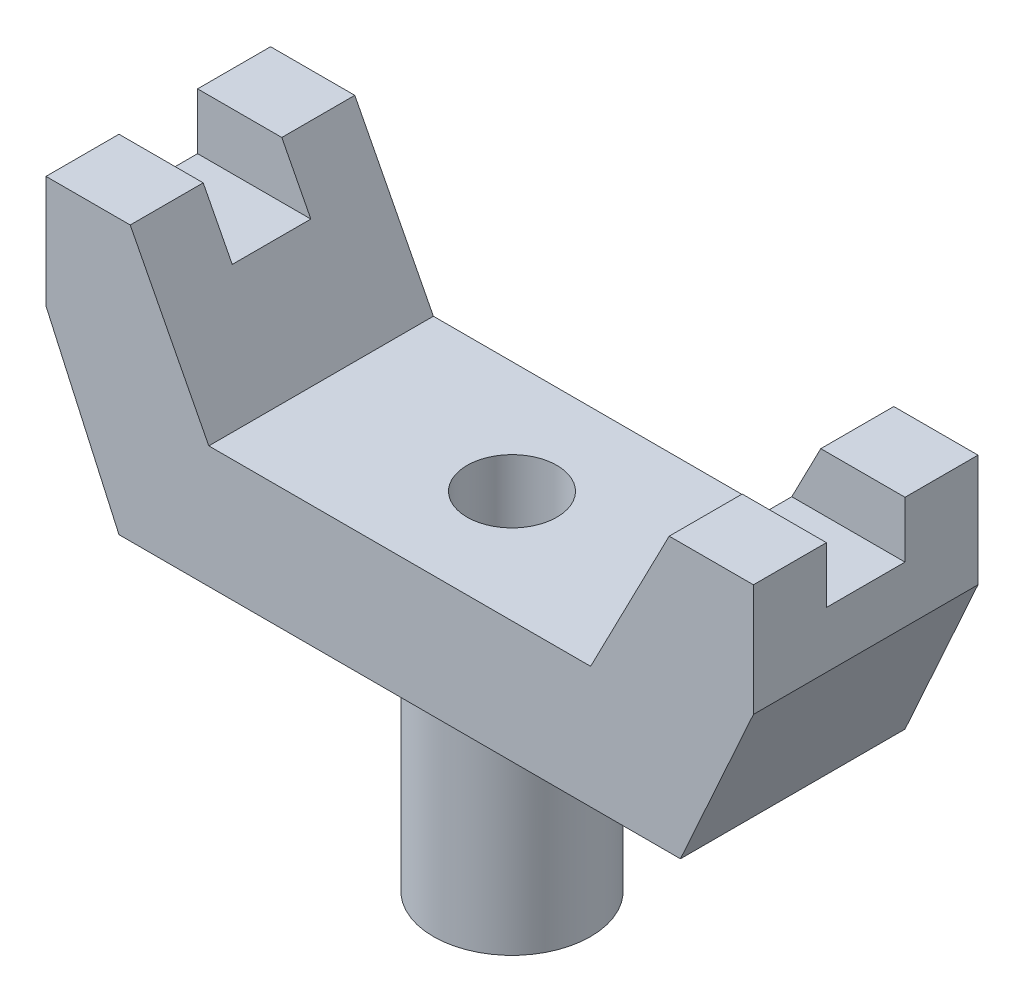
ISO-10303-21;
HEADER;
FILE_DESCRIPTION(('STEP AP214'),'2;1');
FILE_NAME('part.step','',(''),(''),'','','');
FILE_SCHEMA(('AUTOMOTIVE_DESIGN { 1 0 10303 214 1 1 1 1 }'));
ENDSEC;
DATA;
#1=APPLICATION_CONTEXT('core data for automotive mechanical design processes');
#2=APPLICATION_PROTOCOL_DEFINITION('international standard','automotive_design',2000,#1);
#3=PRODUCT_CONTEXT('',#1,'mechanical');
#4=PRODUCT('Part','Part','',(#3));
#5=PRODUCT_RELATED_PRODUCT_CATEGORY('part','',(#4));
#6=PRODUCT_DEFINITION_FORMATION('','',#4);
#7=PRODUCT_DEFINITION_CONTEXT('part definition',#1,'design');
#8=PRODUCT_DEFINITION('design','',#6,#7);
#9=PRODUCT_DEFINITION_SHAPE('','',#8);
#10=(LENGTH_UNIT() NAMED_UNIT(*) SI_UNIT(.MILLI.,.METRE.));
#11=(NAMED_UNIT(*) PLANE_ANGLE_UNIT() SI_UNIT($,.RADIAN.));
#12=(NAMED_UNIT(*) SI_UNIT($,.STERADIAN.) SOLID_ANGLE_UNIT());
#13=UNCERTAINTY_MEASURE_WITH_UNIT(LENGTH_MEASURE(1.E-05),#10,'distance_accuracy_value','');
#14=(GEOMETRIC_REPRESENTATION_CONTEXT(3) GLOBAL_UNCERTAINTY_ASSIGNED_CONTEXT((#13)) GLOBAL_UNIT_ASSIGNED_CONTEXT((#10,
#11,#12)) REPRESENTATION_CONTEXT('',''));
#15=CARTESIAN_POINT('',(0.,0.,0.));
#16=DIRECTION('',(0.,0.,1.));
#17=DIRECTION('',(1.,0.,0.));
#18=AXIS2_PLACEMENT_3D('',#15,#16,#17);
#19=CARTESIAN_POINT('',(-24.,13.5374480416837,10.));
#20=DIRECTION('',(0.,-1.,0.));
#21=DIRECTION('',(1.,0.,0.));
#22=AXIS2_PLACEMENT_3D('',#19,#20,#21);
#23=PLANE('',#22);
#24=DIRECTION('',(0.,0.,-1.));
#25=VECTOR('',#24,1.);
#26=CARTESIAN_POINT('',(-24.,13.5374480416837,10.));
#27=LINE('',#26,#25);
#28=CARTESIAN_POINT('',(-24.,13.5374480416837,10.));
#29=VERTEX_POINT('',#28);
#30=CARTESIAN_POINT('',(-24.,13.5374480416838,3.5));
#31=VERTEX_POINT('',#30);
#32=EDGE_CURVE('E215',#29,#31,#27,.T.);
#33=ORIENTED_EDGE('',*,*,#32,.T.);
#34=DIRECTION('',(-1.,0.,0.));
#35=VECTOR('',#34,1.);
#36=CARTESIAN_POINT('',(31.5,13.5374480416838,3.5));
#37=LINE('',#36,#35);
#38=CARTESIAN_POINT('',(-31.5,13.5374480416838,3.5));
#39=VERTEX_POINT('',#38);
#40=EDGE_CURVE('E238',#31,#39,#37,.T.);
#41=ORIENTED_EDGE('',*,*,#40,.T.);
#42=DIRECTION('',(0.,0.,-1.));
#43=VECTOR('',#42,1.);
#44=CARTESIAN_POINT('',(-31.5,13.5374480416838,10.));
#45=LINE('',#44,#43);
#46=CARTESIAN_POINT('',(-31.5,13.5374480416838,10.));
#47=VERTEX_POINT('',#46);
#48=EDGE_CURVE('E208',#47,#39,#45,.T.);
#49=ORIENTED_EDGE('',*,*,#48,.F.);
#50=DIRECTION('',(-1.,0.,0.));
#51=VECTOR('',#50,1.);
#52=CARTESIAN_POINT('',(-24.,13.5374480416837,10.));
#53=LINE('',#52,#51);
#54=EDGE_CURVE('E262',#29,#47,#53,.T.);
#55=ORIENTED_EDGE('',*,*,#54,.F.);
#56=EDGE_LOOP('',(#33,#41,#49,#55));
#57=FACE_BOUND('',#56,.T.);
#58=ADVANCED_FACE('F39',(#57),#23,.F.);
#59=CARTESIAN_POINT('',(24.,13.5374480416837,10.));
#60=DIRECTION('',(0.,-1.,0.));
#61=DIRECTION('',(1.,0.,0.));
#62=AXIS2_PLACEMENT_3D('',#59,#60,#61);
#63=PLANE('',#62);
#64=DIRECTION('',(0.,0.,-1.));
#65=VECTOR('',#64,1.);
#66=CARTESIAN_POINT('',(31.5,13.5374480416837,10.));
#67=LINE('',#66,#65);
#68=CARTESIAN_POINT('',(31.5,13.5374480416837,10.));
#69=VERTEX_POINT('',#68);
#70=CARTESIAN_POINT('',(31.5,13.5374480416838,3.5));
#71=VERTEX_POINT('',#70);
#72=EDGE_CURVE('E190',#69,#71,#67,.T.);
#73=ORIENTED_EDGE('',*,*,#72,.T.);
#74=CARTESIAN_POINT('',(24.,13.5374480416838,3.5));
#75=VERTEX_POINT('',#74);
#76=EDGE_CURVE('E235',#71,#75,#37,.T.);
#77=ORIENTED_EDGE('',*,*,#76,.T.);
#78=DIRECTION('',(0.,0.,-1.));
#79=VECTOR('',#78,1.);
#80=CARTESIAN_POINT('',(24.,13.5374480416837,10.));
#81=LINE('',#80,#79);
#82=CARTESIAN_POINT('',(24.,13.5374480416837,10.));
#83=VERTEX_POINT('',#82);
#84=EDGE_CURVE('E186',#83,#75,#81,.T.);
#85=ORIENTED_EDGE('',*,*,#84,.F.);
#86=DIRECTION('',(-1.,0.,0.));
#87=VECTOR('',#86,1.);
#88=CARTESIAN_POINT('',(24.,13.5374480416837,10.));
#89=LINE('',#88,#87);
#90=EDGE_CURVE('E277',#69,#83,#89,.T.);
#91=ORIENTED_EDGE('',*,*,#90,.F.);
#92=EDGE_LOOP('',(#73,#77,#85,#91));
#93=FACE_BOUND('',#92,.T.);
#94=ADVANCED_FACE('F237',(#93),#63,.F.);
#95=CARTESIAN_POINT('',(-17.,0.,10.));
#96=DIRECTION('',(-0.888274623195491,-0.459312740719119,0.));
#97=DIRECTION('',(0.459312740719119,-0.888274623195491,0.));
#98=AXIS2_PLACEMENT_3D('',#95,#96,#97);
#99=PLANE('',#98);
#100=DIRECTION('',(0.,0.,1.));
#101=VECTOR('',#100,1.);
#102=CARTESIAN_POINT('',(-21.414579181229,8.53744804168376,10.));
#103=LINE('',#102,#101);
#104=CARTESIAN_POINT('',(-21.414579181229,8.53744804168376,-3.5));
#105=VERTEX_POINT('',#104);
#106=CARTESIAN_POINT('',(-21.414579181229,8.53744804168376,3.5));
#107=VERTEX_POINT('',#106);
#108=EDGE_CURVE('E245',#105,#107,#103,.T.);
#109=ORIENTED_EDGE('',*,*,#108,.T.);
#110=DIRECTION('',(-0.459312740719119,0.888274623195491,0.));
#111=VECTOR('',#110,1.);
#112=CARTESIAN_POINT('',(-17.,0.,3.5));
#113=LINE('',#112,#111);
#114=EDGE_CURVE('E255',#107,#31,#113,.T.);
#115=ORIENTED_EDGE('',*,*,#114,.T.);
#116=ORIENTED_EDGE('',*,*,#32,.F.);
#117=DIRECTION('',(-0.459312740719119,0.888274623195491,0.));
#118=VECTOR('',#117,1.);
#119=CARTESIAN_POINT('',(-17.,0.,10.));
#120=LINE('',#119,#118);
#121=CARTESIAN_POINT('',(-17.,0.,10.));
#122=VERTEX_POINT('',#121);
#123=EDGE_CURVE('E261',#122,#29,#120,.T.);
#124=ORIENTED_EDGE('',*,*,#123,.F.);
#125=DIRECTION('',(0.,0.,-1.));
#126=VECTOR('',#125,1.);
#127=CARTESIAN_POINT('',(-17.,0.,10.));
#128=LINE('',#127,#126);
#129=CARTESIAN_POINT('',(-17.,0.,-10.));
#130=VERTEX_POINT('',#129);
#131=EDGE_CURVE('E214',#122,#130,#128,.T.);
#132=ORIENTED_EDGE('',*,*,#131,.T.);
#133=DIRECTION('',(-0.459312740719119,0.888274623195491,0.));
#134=VECTOR('',#133,1.);
#135=CARTESIAN_POINT('',(-17.,0.,-10.));
#136=LINE('',#135,#134);
#137=CARTESIAN_POINT('',(-24.,13.5374480416837,-10.));
#138=VERTEX_POINT('',#137);
#139=EDGE_CURVE('E260',#130,#138,#136,.T.);
#140=ORIENTED_EDGE('',*,*,#139,.T.);
#141=CARTESIAN_POINT('',(-24.,13.5374480416838,-3.5));
#142=VERTEX_POINT('',#141);
#143=EDGE_CURVE('E211',#142,#138,#27,.T.);
#144=ORIENTED_EDGE('',*,*,#143,.F.);
#145=DIRECTION('',(0.459312740719119,-0.888274623195491,0.));
#146=VECTOR('',#145,1.);
#147=CARTESIAN_POINT('',(-17.,0.,-3.5));
#148=LINE('',#147,#146);
#149=EDGE_CURVE('E239',#142,#105,#148,.T.);
#150=ORIENTED_EDGE('',*,*,#149,.T.);
#151=EDGE_LOOP('',(#109,#115,#116,#124,#132,#140,#144,#150));
#152=FACE_BOUND('',#151,.T.);
#153=ADVANCED_FACE('F41',(#152),#99,.F.);
#154=CARTESIAN_POINT('',(-31.5,13.5374480416838,-3.5));
#155=VERTEX_POINT('',#154);
#156=CARTESIAN_POINT('',(-31.5,13.5374480416838,-10.));
#157=VERTEX_POINT('',#156);
#158=EDGE_CURVE('E210',#155,#157,#45,.T.);
#159=ORIENTED_EDGE('',*,*,#158,.F.);
#160=DIRECTION('',(-1.,0.,0.));
#161=VECTOR('',#160,1.);
#162=CARTESIAN_POINT('',(31.5,13.5374480416838,-3.5));
#163=LINE('',#162,#161);
#164=EDGE_CURVE('E53',#142,#155,#163,.T.);
#165=ORIENTED_EDGE('',*,*,#164,.F.);
#166=ORIENTED_EDGE('',*,*,#143,.T.);
#167=DIRECTION('',(-1.,0.,0.));
#168=VECTOR('',#167,1.);
#169=CARTESIAN_POINT('',(-24.,13.5374480416837,-10.));
#170=LINE('',#169,#168);
#171=EDGE_CURVE('E281',#138,#157,#170,.T.);
#172=ORIENTED_EDGE('',*,*,#171,.T.);
#173=EDGE_LOOP('',(#159,#165,#166,#172));
#174=FACE_BOUND('',#173,.T.);
#175=ADVANCED_FACE('F358',(#174),#23,.F.);
#176=CARTESIAN_POINT('',(-31.5,3.53744804168376,10.));
#177=DIRECTION('',(1.,0.,0.));
#178=DIRECTION('',(0.,0.,-1.));
#179=AXIS2_PLACEMENT_3D('',#176,#177,#178);
#180=PLANE('',#179);
#181=ORIENTED_EDGE('',*,*,#48,.T.);
#182=DIRECTION('',(0.,1.,0.));
#183=VECTOR('',#182,1.);
#184=CARTESIAN_POINT('',(-31.5,13.5374480416838,3.5));
#185=LINE('',#184,#183);
#186=CARTESIAN_POINT('',(-31.5,8.53744804168376,3.5));
#187=VERTEX_POINT('',#186);
#188=EDGE_CURVE('E174',#187,#39,#185,.T.);
#189=ORIENTED_EDGE('',*,*,#188,.F.);
#190=DIRECTION('',(0.,0.,1.));
#191=VECTOR('',#190,1.);
#192=CARTESIAN_POINT('',(-31.5,8.53744804168376,3.5));
#193=LINE('',#192,#191);
#194=CARTESIAN_POINT('',(-31.5,8.53744804168376,-3.5));
#195=VERTEX_POINT('',#194);
#196=EDGE_CURVE('E324',#195,#187,#193,.T.);
#197=ORIENTED_EDGE('',*,*,#196,.F.);
#198=DIRECTION('',(0.,-1.,0.));
#199=VECTOR('',#198,1.);
#200=CARTESIAN_POINT('',(-31.5,8.53744804168376,-3.5));
#201=LINE('',#200,#199);
#202=EDGE_CURVE('E322',#155,#195,#201,.T.);
#203=ORIENTED_EDGE('',*,*,#202,.F.);
#204=ORIENTED_EDGE('',*,*,#158,.T.);
#205=DIRECTION('',(0.,-1.,0.));
#206=VECTOR('',#205,1.);
#207=CARTESIAN_POINT('',(-31.5,3.53744804168376,-10.));
#208=LINE('',#207,#206);
#209=CARTESIAN_POINT('',(-31.5,3.53744804168376,-10.));
#210=VERTEX_POINT('',#209);
#211=EDGE_CURVE('E290',#157,#210,#208,.T.);
#212=ORIENTED_EDGE('',*,*,#211,.T.);
#213=DIRECTION('',(0.,0.,-1.));
#214=VECTOR('',#213,1.);
#215=CARTESIAN_POINT('',(-31.5,3.53744804168376,10.));
#216=LINE('',#215,#214);
#217=CARTESIAN_POINT('',(-31.5,3.53744804168376,10.));
#218=VERTEX_POINT('',#217);
#219=EDGE_CURVE('E204',#218,#210,#216,.T.);
#220=ORIENTED_EDGE('',*,*,#219,.F.);
#221=DIRECTION('',(0.,-1.,0.));
#222=VECTOR('',#221,1.);
#223=CARTESIAN_POINT('',(-31.5,3.53744804168376,10.));
#224=LINE('',#223,#222);
#225=EDGE_CURVE('E266',#47,#218,#224,.T.);
#226=ORIENTED_EDGE('',*,*,#225,.F.);
#227=EDGE_LOOP('',(#181,#189,#197,#203,#204,#212,#220,#226));
#228=FACE_BOUND('',#227,.T.);
#229=ADVANCED_FACE('F340',(#228),#180,.F.);
#230=CARTESIAN_POINT('',(-25.,-10.8483599412518,10.));
#231=DIRECTION('',(0.911294938474,0.41175421687175,0.));
#232=DIRECTION('',(-0.41175421687175,0.911294938474,0.));
#233=AXIS2_PLACEMENT_3D('',#230,#231,#232);
#234=PLANE('',#233);
#235=DIRECTION('',(0.411754216871751,-0.911294938474,0.));
#236=VECTOR('',#235,1.);
#237=CARTESIAN_POINT('',(-25.,-10.8483599412518,-10.));
#238=LINE('',#237,#236);
#239=CARTESIAN_POINT('',(-25.,-10.8483599412518,-10.));
#240=VERTEX_POINT('',#239);
#241=EDGE_CURVE('E289',#210,#240,#238,.T.);
#242=ORIENTED_EDGE('',*,*,#241,.T.);
#243=DIRECTION('',(0.,0.,-1.));
#244=VECTOR('',#243,1.);
#245=CARTESIAN_POINT('',(-25.,-10.8483599412518,10.));
#246=LINE('',#245,#244);
#247=CARTESIAN_POINT('',(-25.,-10.8483599412518,10.));
#248=VERTEX_POINT('',#247);
#249=EDGE_CURVE('E203',#248,#240,#246,.T.);
#250=ORIENTED_EDGE('',*,*,#249,.F.);
#251=DIRECTION('',(0.411754216871751,-0.911294938474,0.));
#252=VECTOR('',#251,1.);
#253=CARTESIAN_POINT('',(-25.,-10.8483599412518,10.));
#254=LINE('',#253,#252);
#255=EDGE_CURVE('E268',#218,#248,#254,.T.);
#256=ORIENTED_EDGE('',*,*,#255,.F.);
#257=ORIENTED_EDGE('',*,*,#219,.T.);
#258=EDGE_LOOP('',(#242,#250,#256,#257));
#259=FACE_BOUND('',#258,.T.);
#260=ADVANCED_FACE('F342',(#259),#234,.F.);
#261=CARTESIAN_POINT('',(-25.,-10.8483599412518,10.));
#262=DIRECTION('',(0.,1.,0.));
#263=DIRECTION('',(0.,0.,1.));
#264=AXIS2_PLACEMENT_3D('',#261,#262,#263);
#265=PLANE('',#264);
#266=CARTESIAN_POINT('',(0.,-10.8483599412518,0.));
#267=DIRECTION('',(0.,1.,0.));
#268=DIRECTION('',(0.,0.,1.));
#269=AXIS2_PLACEMENT_3D('',#266,#267,#268);
#270=CIRCLE('',#269,7.);
#271=CARTESIAN_POINT('',(0.,-10.8483599412518,7.));
#272=VERTEX_POINT('',#271);
#273=EDGE_CURVE('E11',#272,#272,#270,.F.);
#274=ORIENTED_EDGE('',*,*,#273,.F.);
#275=EDGE_LOOP('',(#274));
#276=FACE_BOUND('',#275,.T.);
#277=DIRECTION('',(1.,0.,0.));
#278=VECTOR('',#277,1.);
#279=CARTESIAN_POINT('',(-25.,-10.8483599412518,-10.));
#280=LINE('',#279,#278);
#281=CARTESIAN_POINT('',(25.,-10.8483599412518,-10.));
#282=VERTEX_POINT('',#281);
#283=EDGE_CURVE('E292',#240,#282,#280,.T.);
#284=ORIENTED_EDGE('',*,*,#283,.T.);
#285=DIRECTION('',(0.,0.,-1.));
#286=VECTOR('',#285,1.);
#287=CARTESIAN_POINT('',(25.,-10.8483599412518,10.));
#288=LINE('',#287,#286);
#289=CARTESIAN_POINT('',(25.,-10.8483599412518,10.));
#290=VERTEX_POINT('',#289);
#291=EDGE_CURVE('E196',#290,#282,#288,.T.);
#292=ORIENTED_EDGE('',*,*,#291,.F.);
#293=DIRECTION('',(1.,0.,0.));
#294=VECTOR('',#293,1.);
#295=CARTESIAN_POINT('',(-25.,-10.8483599412518,10.));
#296=LINE('',#295,#294);
#297=EDGE_CURVE('E269',#248,#290,#296,.T.);
#298=ORIENTED_EDGE('',*,*,#297,.F.);
#299=ORIENTED_EDGE('',*,*,#249,.T.);
#300=EDGE_LOOP('',(#284,#292,#298,#299));
#301=FACE_BOUND('',#300,.T.);
#302=ADVANCED_FACE('F349',(#276,#301),#265,.F.);
#303=CARTESIAN_POINT('',(25.,-10.8483599412518,10.));
#304=DIRECTION('',(-0.911294938474,0.41175421687175,0.));
#305=DIRECTION('',(-0.41175421687175,-0.911294938474,0.));
#306=AXIS2_PLACEMENT_3D('',#303,#304,#305);
#307=PLANE('',#306);
#308=DIRECTION('',(0.411754216871751,0.911294938474,0.));
#309=VECTOR('',#308,1.);
#310=CARTESIAN_POINT('',(25.,-10.8483599412518,-10.));
#311=LINE('',#310,#309);
#312=CARTESIAN_POINT('',(31.5,3.53744804168376,-10.));
#313=VERTEX_POINT('',#312);
#314=EDGE_CURVE('E291',#282,#313,#311,.T.);
#315=ORIENTED_EDGE('',*,*,#314,.T.);
#316=DIRECTION('',(0.,0.,-1.));
#317=VECTOR('',#316,1.);
#318=CARTESIAN_POINT('',(31.5,3.53744804168376,10.));
#319=LINE('',#318,#317);
#320=CARTESIAN_POINT('',(31.5,3.53744804168376,10.));
#321=VERTEX_POINT('',#320);
#322=EDGE_CURVE('E195',#321,#313,#319,.T.);
#323=ORIENTED_EDGE('',*,*,#322,.F.);
#324=DIRECTION('',(0.411754216871751,0.911294938474,0.));
#325=VECTOR('',#324,1.);
#326=CARTESIAN_POINT('',(25.,-10.8483599412518,10.));
#327=LINE('',#326,#325);
#328=EDGE_CURVE('E275',#290,#321,#327,.T.);
#329=ORIENTED_EDGE('',*,*,#328,.F.);
#330=ORIENTED_EDGE('',*,*,#291,.T.);
#331=EDGE_LOOP('',(#315,#323,#329,#330));
#332=FACE_BOUND('',#331,.T.);
#333=ADVANCED_FACE('F354',(#332),#307,.F.);
#334=CARTESIAN_POINT('',(31.5,13.5374480416837,10.));
#335=DIRECTION('',(-1.,0.,0.));
#336=DIRECTION('',(0.,0.,1.));
#337=AXIS2_PLACEMENT_3D('',#334,#335,#336);
#338=PLANE('',#337);
#339=DIRECTION('',(0.,0.,1.));
#340=VECTOR('',#339,1.);
#341=CARTESIAN_POINT('',(31.5,8.53744804168376,3.5));
#342=LINE('',#341,#340);
#343=CARTESIAN_POINT('',(31.5,8.53744804168376,-3.5));
#344=VERTEX_POINT('',#343);
#345=CARTESIAN_POINT('',(31.5,8.53744804168376,3.5));
#346=VERTEX_POINT('',#345);
#347=EDGE_CURVE('E172',#344,#346,#342,.T.);
#348=ORIENTED_EDGE('',*,*,#347,.T.);
#349=DIRECTION('',(0.,1.,0.));
#350=VECTOR('',#349,1.);
#351=CARTESIAN_POINT('',(31.5,13.5374480416838,3.5));
#352=LINE('',#351,#350);
#353=EDGE_CURVE('E319',#346,#71,#352,.T.);
#354=ORIENTED_EDGE('',*,*,#353,.T.);
#355=ORIENTED_EDGE('',*,*,#72,.F.);
#356=DIRECTION('',(0.,1.,0.));
#357=VECTOR('',#356,1.);
#358=CARTESIAN_POINT('',(31.5,13.5374480416837,10.));
#359=LINE('',#358,#357);
#360=EDGE_CURVE('E273',#321,#69,#359,.T.);
#361=ORIENTED_EDGE('',*,*,#360,.F.);
#362=ORIENTED_EDGE('',*,*,#322,.T.);
#363=DIRECTION('',(0.,1.,0.));
#364=VECTOR('',#363,1.);
#365=CARTESIAN_POINT('',(31.5,13.5374480416837,-10.));
#366=LINE('',#365,#364);
#367=CARTESIAN_POINT('',(31.5,13.5374480416837,-10.));
#368=VERTEX_POINT('',#367);
#369=EDGE_CURVE('E187',#313,#368,#366,.T.);
#370=ORIENTED_EDGE('',*,*,#369,.T.);
#371=CARTESIAN_POINT('',(31.5,13.5374480416838,-3.5));
#372=VERTEX_POINT('',#371);
#373=EDGE_CURVE('E176',#372,#368,#67,.T.);
#374=ORIENTED_EDGE('',*,*,#373,.F.);
#375=DIRECTION('',(0.,-1.,0.));
#376=VECTOR('',#375,1.);
#377=CARTESIAN_POINT('',(31.5,8.53744804168376,-3.5));
#378=LINE('',#377,#376);
#379=EDGE_CURVE('E162',#372,#344,#378,.T.);
#380=ORIENTED_EDGE('',*,*,#379,.T.);
#381=EDGE_LOOP('',(#348,#354,#355,#361,#362,#370,#374,#380));
#382=FACE_BOUND('',#381,.T.);
#383=ADVANCED_FACE('F181',(#382),#338,.F.);
#384=CARTESIAN_POINT('',(24.,13.5374480416837,-3.5));
#385=VERTEX_POINT('',#384);
#386=CARTESIAN_POINT('',(24.,13.5374480416837,-10.));
#387=VERTEX_POINT('',#386);
#388=EDGE_CURVE('E177',#385,#387,#81,.T.);
#389=ORIENTED_EDGE('',*,*,#388,.F.);
#390=EDGE_CURVE('E64',#372,#385,#163,.T.);
#391=ORIENTED_EDGE('',*,*,#390,.F.);
#392=ORIENTED_EDGE('',*,*,#373,.T.);
#393=DIRECTION('',(-1.,0.,0.));
#394=VECTOR('',#393,1.);
#395=CARTESIAN_POINT('',(24.,13.5374480416837,-10.));
#396=LINE('',#395,#394);
#397=EDGE_CURVE('E297',#368,#387,#396,.T.);
#398=ORIENTED_EDGE('',*,*,#397,.T.);
#399=EDGE_LOOP('',(#389,#391,#392,#398));
#400=FACE_BOUND('',#399,.T.);
#401=ADVANCED_FACE('F178',(#400),#63,.F.);
#402=CARTESIAN_POINT('',(17.,0.,10.));
#403=DIRECTION('',(0.888274623195491,-0.459312740719119,0.));
#404=DIRECTION('',(0.459312740719119,0.888274623195491,0.));
#405=AXIS2_PLACEMENT_3D('',#402,#403,#404);
#406=PLANE('',#405);
#407=ORIENTED_EDGE('',*,*,#84,.T.);
#408=DIRECTION('',(-0.459312740719119,-0.888274623195491,0.));
#409=VECTOR('',#408,1.);
#410=CARTESIAN_POINT('',(17.,0.,3.5));
#411=LINE('',#410,#409);
#412=CARTESIAN_POINT('',(21.414579181229,8.53744804168376,3.5));
#413=VERTEX_POINT('',#412);
#414=EDGE_CURVE('E50',#75,#413,#411,.T.);
#415=ORIENTED_EDGE('',*,*,#414,.T.);
#416=DIRECTION('',(0.,0.,-1.));
#417=VECTOR('',#416,1.);
#418=CARTESIAN_POINT('',(21.414579181229,8.53744804168376,10.));
#419=LINE('',#418,#417);
#420=CARTESIAN_POINT('',(21.414579181229,8.53744804168377,-3.5));
#421=VERTEX_POINT('',#420);
#422=EDGE_CURVE('E219',#413,#421,#419,.T.);
#423=ORIENTED_EDGE('',*,*,#422,.T.);
#424=DIRECTION('',(0.459312740719119,0.888274623195491,0.));
#425=VECTOR('',#424,1.);
#426=CARTESIAN_POINT('',(17.,0.,-3.5));
#427=LINE('',#426,#425);
#428=EDGE_CURVE('E217',#421,#385,#427,.T.);
#429=ORIENTED_EDGE('',*,*,#428,.T.);
#430=ORIENTED_EDGE('',*,*,#388,.T.);
#431=DIRECTION('',(-0.459312740719119,-0.888274623195491,0.));
#432=VECTOR('',#431,1.);
#433=CARTESIAN_POINT('',(17.,0.,-10.));
#434=LINE('',#433,#432);
#435=CARTESIAN_POINT('',(17.,0.,-10.));
#436=VERTEX_POINT('',#435);
#437=EDGE_CURVE('E300',#387,#436,#434,.T.);
#438=ORIENTED_EDGE('',*,*,#437,.T.);
#439=DIRECTION('',(0.,0.,-1.));
#440=VECTOR('',#439,1.);
#441=CARTESIAN_POINT('',(17.,0.,10.));
#442=LINE('',#441,#440);
#443=CARTESIAN_POINT('',(17.,0.,10.));
#444=VERTEX_POINT('',#443);
#445=EDGE_CURVE('E282',#444,#436,#442,.T.);
#446=ORIENTED_EDGE('',*,*,#445,.F.);
#447=DIRECTION('',(-0.459312740719119,-0.888274623195491,0.));
#448=VECTOR('',#447,1.);
#449=CARTESIAN_POINT('',(17.,0.,10.));
#450=LINE('',#449,#448);
#451=EDGE_CURVE('E279',#83,#444,#450,.T.);
#452=ORIENTED_EDGE('',*,*,#451,.F.);
#453=EDGE_LOOP('',(#407,#415,#423,#429,#430,#438,#446,#452));
#454=FACE_BOUND('',#453,.T.);
#455=ADVANCED_FACE('F221',(#454),#406,.F.);
#456=CARTESIAN_POINT('',(0.,0.,10.));
#457=DIRECTION('',(0.,-1.,0.));
#458=DIRECTION('',(0.,0.,-1.));
#459=AXIS2_PLACEMENT_3D('',#456,#457,#458);
#460=PLANE('',#459);
#461=CARTESIAN_POINT('',(0.,0.,0.));
#462=DIRECTION('',(0.,1.,0.));
#463=DIRECTION('',(0.,0.,1.));
#464=AXIS2_PLACEMENT_3D('',#461,#462,#463);
#465=CIRCLE('',#464,4.);
#466=CARTESIAN_POINT('',(0.,0.,4.));
#467=VERTEX_POINT('',#466);
#468=EDGE_CURVE('E326',#467,#467,#465,.T.);
#469=ORIENTED_EDGE('',*,*,#468,.F.);
#470=EDGE_LOOP('',(#469));
#471=FACE_BOUND('',#470,.T.);
#472=DIRECTION('',(-1.,0.,0.));
#473=VECTOR('',#472,1.);
#474=CARTESIAN_POINT('',(0.,0.,-10.));
#475=LINE('',#474,#473);
#476=EDGE_CURVE('E265',#436,#130,#475,.T.);
#477=ORIENTED_EDGE('',*,*,#476,.T.);
#478=ORIENTED_EDGE('',*,*,#131,.F.);
#479=DIRECTION('',(-1.,0.,0.));
#480=VECTOR('',#479,1.);
#481=CARTESIAN_POINT('',(-17.,0.,10.));
#482=LINE('',#481,#480);
#483=EDGE_CURVE('E256',#444,#122,#482,.T.);
#484=ORIENTED_EDGE('',*,*,#483,.F.);
#485=ORIENTED_EDGE('',*,*,#445,.T.);
#486=EDGE_LOOP('',(#477,#478,#484,#485));
#487=FACE_BOUND('',#486,.T.);
#488=ADVANCED_FACE('F309',(#471,#487),#460,.F.);
#489=CARTESIAN_POINT('',(0.,0.,10.));
#490=DIRECTION('',(0.,0.,-1.));
#491=DIRECTION('',(-1.,0.,0.));
#492=AXIS2_PLACEMENT_3D('',#489,#490,#491);
#493=PLANE('',#492);
#494=ORIENTED_EDGE('',*,*,#483,.T.);
#495=ORIENTED_EDGE('',*,*,#123,.T.);
#496=ORIENTED_EDGE('',*,*,#54,.T.);
#497=ORIENTED_EDGE('',*,*,#225,.T.);
#498=ORIENTED_EDGE('',*,*,#255,.T.);
#499=ORIENTED_EDGE('',*,*,#297,.T.);
#500=ORIENTED_EDGE('',*,*,#328,.T.);
#501=ORIENTED_EDGE('',*,*,#360,.T.);
#502=ORIENTED_EDGE('',*,*,#90,.T.);
#503=ORIENTED_EDGE('',*,*,#451,.T.);
#504=EDGE_LOOP('',(#494,#495,#496,#497,#498,#499,#500,#501,#502,#503));
#505=FACE_BOUND('',#504,.T.);
#506=ADVANCED_FACE('F316',(#505),#493,.F.);
#507=CARTESIAN_POINT('',(0.,0.,-10.));
#508=DIRECTION('',(0.,0.,-1.));
#509=DIRECTION('',(-1.,0.,0.));
#510=AXIS2_PLACEMENT_3D('',#507,#508,#509);
#511=PLANE('',#510);
#512=ORIENTED_EDGE('',*,*,#139,.F.);
#513=ORIENTED_EDGE('',*,*,#476,.F.);
#514=ORIENTED_EDGE('',*,*,#437,.F.);
#515=ORIENTED_EDGE('',*,*,#397,.F.);
#516=ORIENTED_EDGE('',*,*,#369,.F.);
#517=ORIENTED_EDGE('',*,*,#314,.F.);
#518=ORIENTED_EDGE('',*,*,#283,.F.);
#519=ORIENTED_EDGE('',*,*,#241,.F.);
#520=ORIENTED_EDGE('',*,*,#211,.F.);
#521=ORIENTED_EDGE('',*,*,#171,.F.);
#522=EDGE_LOOP('',(#512,#513,#514,#515,#516,#517,#518,#519,#520,#521));
#523=FACE_BOUND('',#522,.T.);
#524=ADVANCED_FACE('F307',(#523),#511,.T.);
#525=CARTESIAN_POINT('',(31.5,8.53744804168376,-3.5));
#526=DIRECTION('',(0.,0.,-1.));
#527=DIRECTION('',(-1.,0.,0.));
#528=AXIS2_PLACEMENT_3D('',#525,#526,#527);
#529=PLANE('',#528);
#530=DIRECTION('',(-1.,0.,0.));
#531=VECTOR('',#530,1.);
#532=CARTESIAN_POINT('',(31.5,8.53744804168376,-3.5));
#533=LINE('',#532,#531);
#534=EDGE_CURVE('E167',#344,#421,#533,.T.);
#535=ORIENTED_EDGE('',*,*,#534,.F.);
#536=ORIENTED_EDGE('',*,*,#379,.F.);
#537=ORIENTED_EDGE('',*,*,#390,.T.);
#538=ORIENTED_EDGE('',*,*,#428,.F.);
#539=EDGE_LOOP('',(#535,#536,#537,#538));
#540=FACE_BOUND('',#539,.T.);
#541=ADVANCED_FACE('F163',(#540),#529,.F.);
#542=CARTESIAN_POINT('',(31.5,8.53744804168376,3.5));
#543=DIRECTION('',(0.,-1.,0.));
#544=DIRECTION('',(0.,0.,-1.));
#545=AXIS2_PLACEMENT_3D('',#542,#543,#544);
#546=PLANE('',#545);
#547=DIRECTION('',(-1.,0.,0.));
#548=VECTOR('',#547,1.);
#549=CARTESIAN_POINT('',(31.5,8.53744804168376,3.5));
#550=LINE('',#549,#548);
#551=EDGE_CURVE('E234',#346,#413,#550,.T.);
#552=ORIENTED_EDGE('',*,*,#551,.F.);
#553=ORIENTED_EDGE('',*,*,#347,.F.);
#554=ORIENTED_EDGE('',*,*,#534,.T.);
#555=ORIENTED_EDGE('',*,*,#422,.F.);
#556=EDGE_LOOP('',(#552,#553,#554,#555));
#557=FACE_BOUND('',#556,.T.);
#558=ADVANCED_FACE('F362',(#557),#546,.F.);
#559=CARTESIAN_POINT('',(31.5,13.5374480416838,3.5));
#560=DIRECTION('',(0.,0.,1.));
#561=DIRECTION('',(0.,-1.,0.));
#562=AXIS2_PLACEMENT_3D('',#559,#560,#561);
#563=PLANE('',#562);
#564=ORIENTED_EDGE('',*,*,#76,.F.);
#565=ORIENTED_EDGE('',*,*,#353,.F.);
#566=ORIENTED_EDGE('',*,*,#551,.T.);
#567=ORIENTED_EDGE('',*,*,#414,.F.);
#568=EDGE_LOOP('',(#564,#565,#566,#567));
#569=FACE_BOUND('',#568,.T.);
#570=ADVANCED_FACE('F228',(#569),#563,.F.);
#571=EDGE_CURVE('E247',#107,#187,#550,.T.);
#572=ORIENTED_EDGE('',*,*,#571,.T.);
#573=ORIENTED_EDGE('',*,*,#188,.T.);
#574=ORIENTED_EDGE('',*,*,#40,.F.);
#575=ORIENTED_EDGE('',*,*,#114,.F.);
#576=EDGE_LOOP('',(#572,#573,#574,#575));
#577=FACE_BOUND('',#576,.T.);
#578=ADVANCED_FACE('F334',(#577),#563,.F.);
#579=EDGE_CURVE('E182',#105,#195,#533,.T.);
#580=ORIENTED_EDGE('',*,*,#579,.T.);
#581=ORIENTED_EDGE('',*,*,#196,.T.);
#582=ORIENTED_EDGE('',*,*,#571,.F.);
#583=ORIENTED_EDGE('',*,*,#108,.F.);
#584=EDGE_LOOP('',(#580,#581,#582,#583));
#585=FACE_BOUND('',#584,.T.);
#586=ADVANCED_FACE('F359',(#585),#546,.F.);
#587=ORIENTED_EDGE('',*,*,#164,.T.);
#588=ORIENTED_EDGE('',*,*,#202,.T.);
#589=ORIENTED_EDGE('',*,*,#579,.F.);
#590=ORIENTED_EDGE('',*,*,#149,.F.);
#591=EDGE_LOOP('',(#587,#588,#589,#590));
#592=FACE_BOUND('',#591,.T.);
#593=ADVANCED_FACE('F356',(#592),#529,.F.);
#594=CARTESIAN_POINT('',(0.,-20.,0.));
#595=DIRECTION('',(0.,1.,0.));
#596=DIRECTION('',(0.,0.,1.));
#597=AXIS2_PLACEMENT_3D('',#594,#595,#596);
#598=CYLINDRICAL_SURFACE('',#597,4.);
#599=ORIENTED_EDGE('',*,*,#468,.T.);
#600=EDGE_LOOP('',(#599));
#601=FACE_BOUND('',#600,.T.);
#602=CARTESIAN_POINT('',(0.,-30.8483599412518,0.));
#603=DIRECTION('',(0.,1.,0.));
#604=DIRECTION('',(0.,0.,1.));
#605=AXIS2_PLACEMENT_3D('',#602,#603,#604);
#606=CIRCLE('',#605,4.);
#607=CARTESIAN_POINT('',(0.,-30.8483599412518,4.));
#608=VERTEX_POINT('',#607);
#609=EDGE_CURVE('E560',#608,#608,#606,.T.);
#610=ORIENTED_EDGE('',*,*,#609,.F.);
#611=EDGE_LOOP('',(#610));
#612=FACE_BOUND('',#611,.T.);
#613=ADVANCED_FACE('F370',(#601,#612),#598,.F.);
#614=CARTESIAN_POINT('',(0.,-30.8483599412518,0.));
#615=DIRECTION('',(0.,1.,0.));
#616=DIRECTION('',(0.,0.,1.));
#617=AXIS2_PLACEMENT_3D('',#614,#615,#616);
#618=CYLINDRICAL_SURFACE('',#617,7.);
#619=CARTESIAN_POINT('',(0.,-30.8483599412518,0.));
#620=DIRECTION('',(0.,-1.,0.));
#621=DIRECTION('',(0.,0.,-1.));
#622=AXIS2_PLACEMENT_3D('',#619,#620,#621);
#623=CIRCLE('',#622,7.);
#624=CARTESIAN_POINT('',(0.,-30.8483599412518,-7.));
#625=VERTEX_POINT('',#624);
#626=EDGE_CURVE('E553',#625,#625,#623,.T.);
#627=ORIENTED_EDGE('',*,*,#626,.F.);
#628=EDGE_LOOP('',(#627));
#629=FACE_BOUND('',#628,.T.);
#630=ORIENTED_EDGE('',*,*,#273,.T.);
#631=EDGE_LOOP('',(#630));
#632=FACE_BOUND('',#631,.T.);
#633=ADVANCED_FACE('F438',(#629,#632),#618,.T.);
#634=CARTESIAN_POINT('',(0.,-30.8483599412518,0.));
#635=DIRECTION('',(0.,-1.,0.));
#636=DIRECTION('',(0.,0.,-1.));
#637=AXIS2_PLACEMENT_3D('',#634,#635,#636);
#638=PLANE('',#637);
#639=ORIENTED_EDGE('',*,*,#609,.T.);
#640=EDGE_LOOP('',(#639));
#641=FACE_BOUND('',#640,.T.);
#642=ORIENTED_EDGE('',*,*,#626,.T.);
#643=EDGE_LOOP('',(#642));
#644=FACE_BOUND('',#643,.T.);
#645=ADVANCED_FACE('F446',(#641,#644),#638,.T.);
#646=CLOSED_SHELL('',(#58,#94,#153,#175,#229,#260,#302,#333,#383,#401,#455,#488,#506,#524,#541,
#558,#570,#578,#586,#593,#613,#633,#645));
#647=MANIFOLD_SOLID_BREP('B2',#646);
#648=ADVANCED_BREP_SHAPE_REPRESENTATION('',(#18,#647),#14);
#649=SHAPE_DEFINITION_REPRESENTATION(#9,#648);
ENDSEC;
END-ISO-10303-21;
